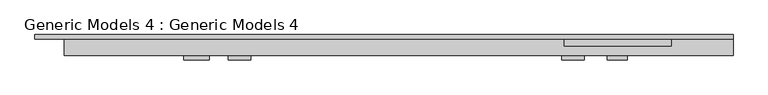
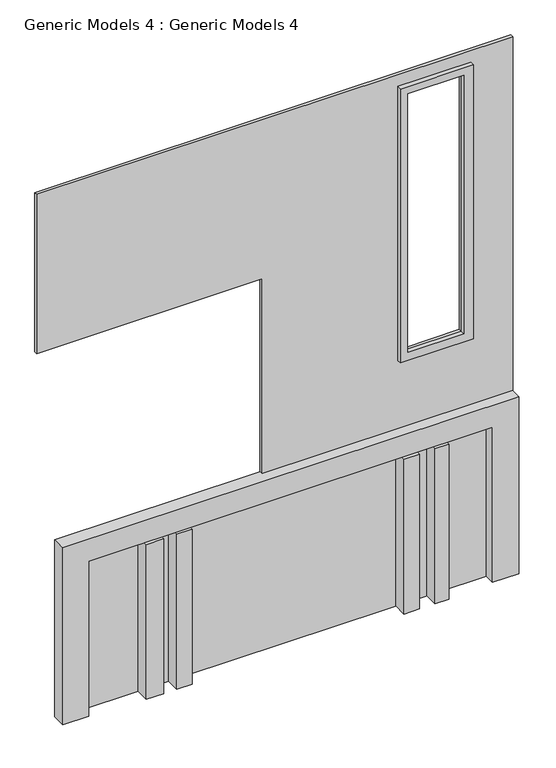
"""IFC4 building model written with IfcOpenShell, lengths in millimetres: proxy geometry, Generic Models 4 : Generic Models 4."""

from ifc_helpers import new_model, si_unit, frame, origin, origin_with_axes, place, context, project, spatial, polyline, outline, extrude, source, transform, mapped, element, save


def generic_models_4_generic_models_4_c94f5d84(model_context):
    return source(origin(), model_context, "Body", "SweptSolid", [
        extrude(outline(polyline([(4227.0998045, -13394.0503587), (8945.9950276, -13394.0503587), (8945.9950276, -14587.8503587), (4227.0998045, -14587.8503587), (4227.0998045, -13394.0503587)]), holes=[polyline([(8818.9950276, -13546.4503587), (4361.7460332, -13546.4503587), (4361.7460332, -14460.8503587), (8818.9950276, -14460.8503587), (8818.9950276, -13546.4503587)])]), frame((0.0, -14000.3526331, 0.0), z_axis=(0.0, 1.0, 0.0), x_axis=(0.0, 0.0, 1.0)), (0.0, 0.0, 1.0), 76.2),
        extrude(outline(polyline([(9144.0, -20474.3003587), (6400.8, -20474.3003587), (6400.8, -16797.6503587), (3048.0, -16797.6503587), (3048.0, -12707.0553745), (9144.0, -12707.0553745), (9144.0, -20474.3003587)]), holes=[polyline([(8818.9950276, -13546.4503587), (4361.7460332, -13546.4503587), (4361.7460332, -14460.8503587), (8818.9950276, -14460.8503587), (8818.9950276, -13546.4503587)])]), frame((0.0, -13924.1526331, 0.0), z_axis=(0.0, 1.0, 0.0), x_axis=(0.0, 0.0, 1.0)), (0.0, 0.0, 1.0), 50.8),
        extrude(outline(polyline([(-14365.6003587, -14152.7526331), (-14613.2503587, -14152.7526331), (-14613.2503587, -13924.1526331), (-14365.6003587, -13924.1526331), (-14365.6003587, -14152.7526331)])), origin_with_axes(), (0.0, 0.0, 1.0), 2669.0215701),
        extrude(outline(polyline([(-13883.0003587, -14152.7526331), (-14108.6835875, -14152.7526331), (-14108.6835875, -13924.1526331), (-13883.0003587, -13924.1526331), (-13883.0003587, -14152.7526331)])), origin_with_axes(), (0.0, 0.0, 1.0), 2669.0215701),
        extrude(outline(polyline([(-18074.0003587, -14152.7526331), (-18321.6503587, -14152.7526331), (-18321.6503587, -13924.1526331), (-18074.0003587, -13924.1526331), (-18074.0003587, -14152.7526331)])), origin_with_axes(), (0.0, 0.0, 1.0), 2669.0215701),
        extrude(outline(polyline([(-18533.8434026, -14152.7526331), (-18818.8452159, -14152.7526331), (-18818.8452159, -13924.1526331), (-18533.8434026, -13924.1526331), (-18533.8434026, -14152.7526331)])), origin_with_axes(), (0.0, 0.0, 1.0), 2669.0215701),
        extrude(outline(polyline([(-13140.0503587, -13924.1526331), (-19731.996137, -13924.1526331), (-19731.996137, -13873.3526331), (-13140.0503587, -13873.3526331), (-13140.0503587, -13924.1526331)])), origin_with_axes(), (0.0, 0.0, 1.0), 2669.0215701),
        extrude(outline(polyline([(3048.0, -20150.4503587), (0.0, -20150.4503587), (0.0, -19731.996137), (2669.0215701, -19731.996137), (2669.0215701, -13140.0503587), (0.0, -13140.0503587), (0.0, -12707.0553745), (3048.0, -12707.0553745), (3048.0, -20150.4503587)])), frame((0.0, -14101.9526331, 0.0), z_axis=(0.0, 1.0, 0.0), x_axis=(0.0, 0.0, 1.0)), (0.0, 0.0, 1.0), 228.6),
    ])


if __name__ == "__main__":
    model = new_model("IFC4")
    model_context = context("Model", 3, world=origin())
    ifc_project = project(units=[si_unit("LENGTHUNIT", "METRE", prefix="MILLI")], contexts=[model_context])
    site = spatial("IfcSite", under=ifc_project)
    building = spatial("IfcBuilding", under=site)
    placement = place(None, origin())
    generic_models_4_generic_models_4_shape = generic_models_4_generic_models_4_c94f5d84(model_context)
    element("IfcBuildingElementProxy", 1, Name="Generic Models 4 : Generic Models 4", ObjectType="Generic Models 4 : Generic Models 4", at=placement, inside=building, context=model_context, shape_type="MappedRepresentation", body=[
        mapped(generic_models_4_generic_models_4_shape, transform((0.0, 0.0, 0.0), x_axis=(1.0, 0.0, 0.0), y_axis=(0.0, 1.0, 0.0), z_axis=(0.0, 0.0, 1.0))),
    ])
    save(model, "model.ifc")
